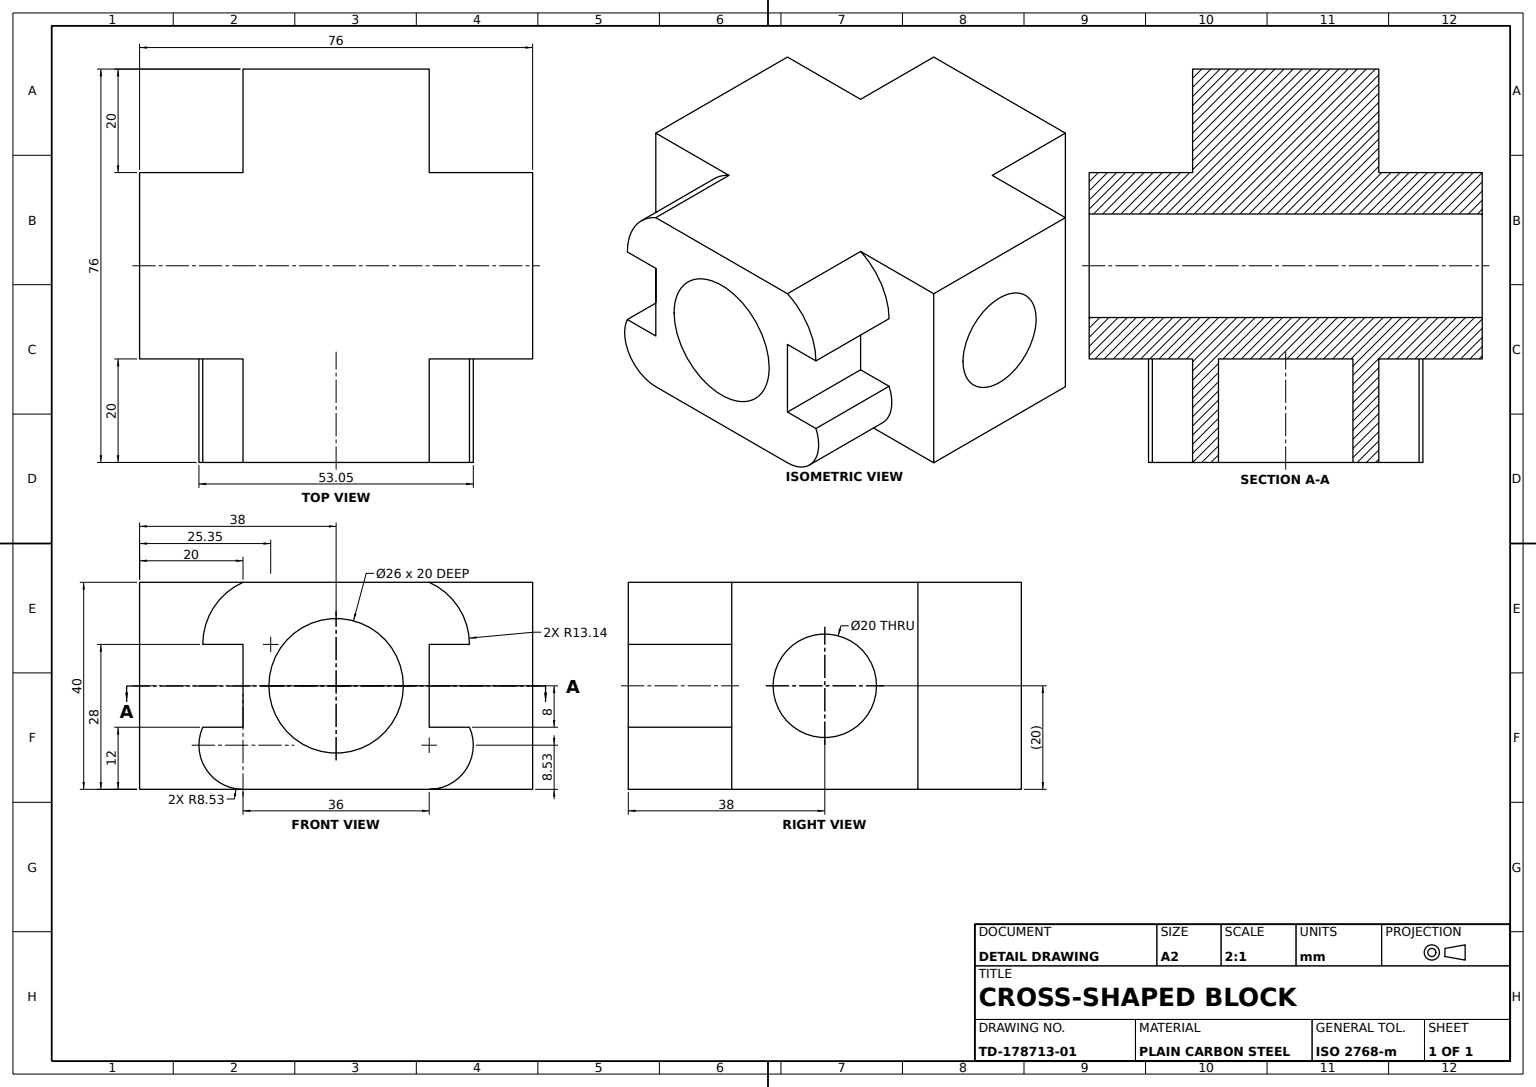
from build123d import *

# Parameters (mm, degrees)
CROSS_BLOCK_DEPTH      = 40
SIDE_LUG_DEPTH         = 20
BORE_26_SKETCH_R       = 13
BORE_26_DEPTH          = 20
CROSS_HOLE_20_SKETCH_R = 10
CROSS_HOLE_20_DEPTH    = 103.528044944


with BuildPart() as part:
    # Cross Profile Sketch → Cross Block (new body)
    with BuildSketch(Plane(origin=(0, 0, 0), x_dir=(1, 0, 0), z_dir=(0, 1, 0))):
        Polygon((0, 0), (20, 0), (20, 20), (56, 20), (56, 0), (76, 0), (76, -36), (56, -36), (56, -56), (20, -56), (20, -36), (0, -36), align=None)
    extrude(amount=CROSS_BLOCK_DEPTH)

    # Side Lug Sketch → Side Lug (add)
    with BuildSketch(Plane.XY.offset(56)):
        with BuildLine():
            Line((12.212406084, 28), (20, 28))
            Line((20, 28), (20, 40))
            ThreePointArc((20, 40), (14.32993543, 35.15273757), (12.212406084, 28))
        make_face()
        with BuildLine():
            Line((56, 40), (56, 28))
            Line((56, 28), (63.787593916, 28))
            ThreePointArc((63.787593916, 28), (61.67006457, 35.15273757), (56, 40))
        make_face()
        with BuildLine():
            Line((63.787593916, 12), (56, 12))
            Line((56, 12), (56, 0))
            ThreePointArc((56, 0), (63.15273757, 3.885057826), (63.787593916, 12))
        make_face()
        with BuildLine():
            Line((20, 0), (20, 12))
            Line((20, 12), (12.212406084, 12))
            ThreePointArc((12.212406084, 12), (12.84726243, 3.885057826), (20, 0))
        make_face()
    extrude(amount=-SIDE_LUG_DEPTH)

    # Bore Ø26 Sketch → Bore Ø26 (cut)
    with BuildSketch(Plane.XY.offset(56)):
        with Locations((38, 20)):
            Circle(BORE_26_SKETCH_R)
    extrude(amount=-BORE_26_DEPTH, mode=Mode.SUBTRACT)

    # Cross Hole Ø20 Sketch → Cross Hole Ø20 (cut, through all)
    with BuildSketch(Plane(origin=(76, 0, 0), x_dir=(0, 0, -1), z_dir=(1, 0, 0))):
        with Locations((-18, 20)):
            Circle(CROSS_HOLE_20_SKETCH_R)
    extrude(amount=-CROSS_HOLE_20_DEPTH, mode=Mode.SUBTRACT)


solid = part.part
